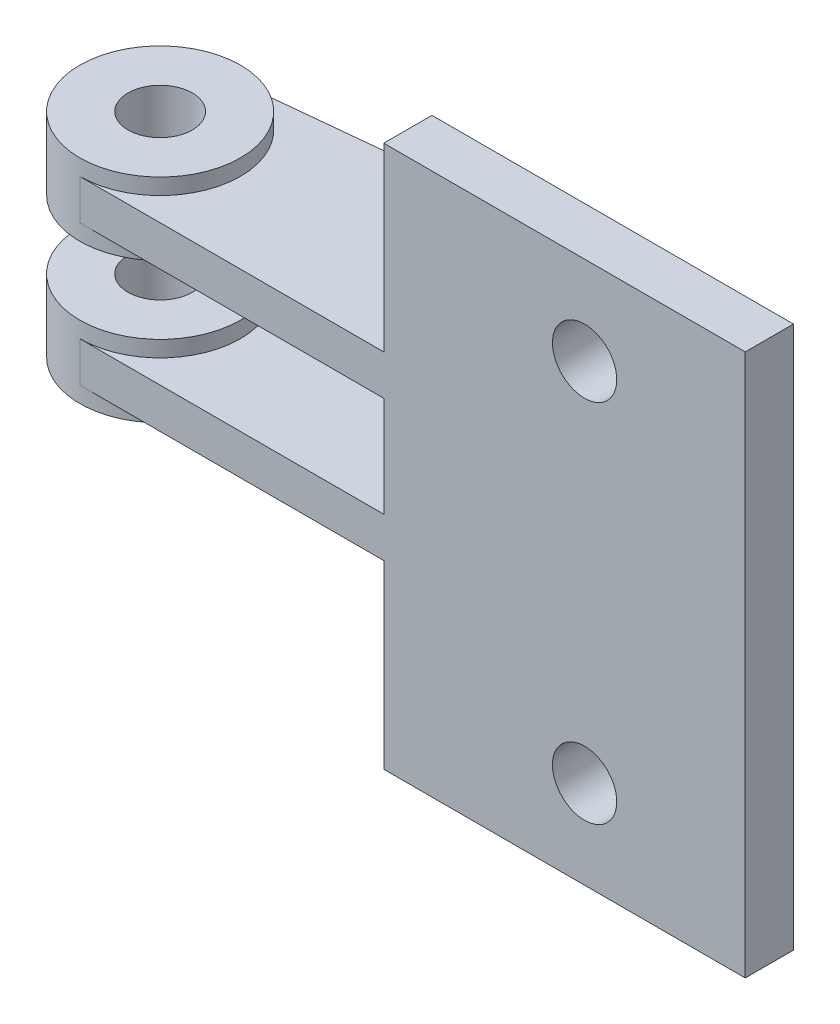
ISO-10303-21;
HEADER;
FILE_DESCRIPTION(('STEP AP214'),'2;1');
FILE_NAME('part.step','',(''),(''),'','','');
FILE_SCHEMA(('AUTOMOTIVE_DESIGN { 1 0 10303 214 1 1 1 1 }'));
ENDSEC;
DATA;
#1=APPLICATION_CONTEXT('core data for automotive mechanical design processes');
#2=APPLICATION_PROTOCOL_DEFINITION('international standard','automotive_design',2000,#1);
#3=PRODUCT_CONTEXT('',#1,'mechanical');
#4=PRODUCT('Part','Part','',(#3));
#5=PRODUCT_RELATED_PRODUCT_CATEGORY('part','',(#4));
#6=PRODUCT_DEFINITION_FORMATION('','',#4);
#7=PRODUCT_DEFINITION_CONTEXT('part definition',#1,'design');
#8=PRODUCT_DEFINITION('design','',#6,#7);
#9=PRODUCT_DEFINITION_SHAPE('','',#8);
#10=(LENGTH_UNIT() NAMED_UNIT(*) SI_UNIT(.MILLI.,.METRE.));
#11=(NAMED_UNIT(*) PLANE_ANGLE_UNIT() SI_UNIT($,.RADIAN.));
#12=(NAMED_UNIT(*) SI_UNIT($,.STERADIAN.) SOLID_ANGLE_UNIT());
#13=UNCERTAINTY_MEASURE_WITH_UNIT(LENGTH_MEASURE(1.E-05),#10,'distance_accuracy_value','');
#14=(GEOMETRIC_REPRESENTATION_CONTEXT(3) GLOBAL_UNCERTAINTY_ASSIGNED_CONTEXT((#13)) GLOBAL_UNIT_ASSIGNED_CONTEXT((#10,
#11,#12)) REPRESENTATION_CONTEXT('',''));
#15=CARTESIAN_POINT('',(0.,0.,0.));
#16=DIRECTION('',(0.,0.,1.));
#17=DIRECTION('',(1.,0.,0.));
#18=AXIS2_PLACEMENT_3D('',#15,#16,#17);
#19=CARTESIAN_POINT('',(-140.672374094552,12.5,0.));
#20=DIRECTION('',(0.,1.,0.));
#21=DIRECTION('',(0.,0.,1.));
#22=AXIS2_PLACEMENT_3D('',#19,#20,#21);
#23=PLANE('',#22);
#24=CARTESIAN_POINT('',(-120.672374094552,12.5,-7.99999999999999));
#25=DIRECTION('',(0.,1.,0.));
#26=DIRECTION('',(0.,0.,1.));
#27=AXIS2_PLACEMENT_3D('',#24,#25,#26);
#28=CIRCLE('',#27,20.);
#29=CARTESIAN_POINT('',(-122.695594955068,12.5,-27.8974012712609));
#30=VERTEX_POINT('',#29);
#31=CARTESIAN_POINT('',(-120.672374094552,12.5,12.));
#32=VERTEX_POINT('',#31);
#33=EDGE_CURVE('E11',#30,#32,#28,.F.);
#34=ORIENTED_EDGE('',*,*,#33,.F.);
#35=DIRECTION('',(-0.994870063563044,0.,0.10116104302579));
#36=VECTOR('',#35,1.);
#37=CARTESIAN_POINT('',(-4.06326518045554,12.5,-39.9602531512327));
#38=LINE('',#37,#36);
#39=CARTESIAN_POINT('',(-3.67237409455184,12.5,-40.));
#40=VERTEX_POINT('',#39);
#41=EDGE_CURVE('E275',#40,#30,#38,.T.);
#42=ORIENTED_EDGE('',*,*,#41,.F.);
#43=DIRECTION('',(-0.772577366580188,0.,-0.634920634920635));
#44=VECTOR('',#43,1.);
#45=CARTESIAN_POINT('',(18.140589569161,12.5,-22.0736390451482));
#46=LINE('',#45,#44);
#47=CARTESIAN_POINT('',(45.,12.5,0.));
#48=VERTEX_POINT('',#47);
#49=EDGE_CURVE('E281',#48,#40,#46,.T.);
#50=ORIENTED_EDGE('',*,*,#49,.F.);
#51=DIRECTION('',(1.,0.,0.));
#52=VECTOR('',#51,1.);
#53=CARTESIAN_POINT('',(-140.672374094552,12.5,0.));
#54=LINE('',#53,#52);
#55=CARTESIAN_POINT('',(-45.,12.5,0.));
#56=VERTEX_POINT('',#55);
#57=EDGE_CURVE('E61',#56,#48,#54,.T.);
#58=ORIENTED_EDGE('',*,*,#57,.F.);
#59=DIRECTION('',(0.,0.,1.));
#60=VECTOR('',#59,1.);
#61=CARTESIAN_POINT('',(-45.,12.5,-40.));
#62=LINE('',#61,#60);
#63=CARTESIAN_POINT('',(-45.,12.5,12.));
#64=VERTEX_POINT('',#63);
#65=EDGE_CURVE('E167',#56,#64,#62,.T.);
#66=ORIENTED_EDGE('',*,*,#65,.T.);
#67=DIRECTION('',(-1.,0.,0.));
#68=VECTOR('',#67,1.);
#69=CARTESIAN_POINT('',(-139.002676874375,12.5,12.));
#70=LINE('',#69,#68);
#71=EDGE_CURVE('E163',#64,#32,#70,.T.);
#72=ORIENTED_EDGE('',*,*,#71,.T.);
#73=EDGE_LOOP('',(#34,#42,#50,#58,#66,#72));
#74=FACE_BOUND('',#73,.T.);
#75=ADVANCED_FACE('F41',(#74),#23,.F.);
#76=CARTESIAN_POINT('',(0.,22.5,0.));
#77=DIRECTION('',(0.,1.,0.));
#78=DIRECTION('',(0.,0.,1.));
#79=AXIS2_PLACEMENT_3D('',#76,#77,#78);
#80=PLANE('',#79);
#81=DIRECTION('',(-0.994870063563044,0.,0.10116104302579));
#82=VECTOR('',#81,1.);
#83=CARTESIAN_POINT('',(-4.06326518045554,22.5,-39.9602531512327));
#84=LINE('',#83,#82);
#85=CARTESIAN_POINT('',(-3.67237409455183,22.5,-40.));
#86=VERTEX_POINT('',#85);
#87=CARTESIAN_POINT('',(-122.695594955068,22.5,-27.8974012712609));
#88=VERTEX_POINT('',#87);
#89=EDGE_CURVE('E270',#86,#88,#84,.T.);
#90=ORIENTED_EDGE('',*,*,#89,.T.);
#91=CARTESIAN_POINT('',(-120.672374094552,22.5,-7.99999999999999));
#92=DIRECTION('',(0.,1.,0.));
#93=DIRECTION('',(0.,0.,1.));
#94=AXIS2_PLACEMENT_3D('',#91,#92,#93);
#95=CIRCLE('',#94,20.);
#96=CARTESIAN_POINT('',(-120.672374094552,22.5,12.));
#97=VERTEX_POINT('',#96);
#98=EDGE_CURVE('E177',#97,#88,#95,.T.);
#99=ORIENTED_EDGE('',*,*,#98,.F.);
#100=DIRECTION('',(-1.,0.,0.));
#101=VECTOR('',#100,1.);
#102=CARTESIAN_POINT('',(0.,22.5,12.));
#103=LINE('',#102,#101);
#104=CARTESIAN_POINT('',(-45.,22.5,12.));
#105=VERTEX_POINT('',#104);
#106=EDGE_CURVE('E161',#105,#97,#103,.T.);
#107=ORIENTED_EDGE('',*,*,#106,.F.);
#108=DIRECTION('',(0.,0.,-1.));
#109=VECTOR('',#108,1.);
#110=CARTESIAN_POINT('',(-45.,22.5,0.));
#111=LINE('',#110,#109);
#112=CARTESIAN_POINT('',(-45.,22.5,0.));
#113=VERTEX_POINT('',#112);
#114=EDGE_CURVE('E279',#105,#113,#111,.T.);
#115=ORIENTED_EDGE('',*,*,#114,.T.);
#116=DIRECTION('',(-1.,0.,0.));
#117=VECTOR('',#116,1.);
#118=CARTESIAN_POINT('',(0.,22.5,0.));
#119=LINE('',#118,#117);
#120=CARTESIAN_POINT('',(45.,22.5,0.));
#121=VERTEX_POINT('',#120);
#122=EDGE_CURVE('E273',#121,#113,#119,.T.);
#123=ORIENTED_EDGE('',*,*,#122,.F.);
#124=DIRECTION('',(-0.772577366580188,0.,-0.634920634920635));
#125=VECTOR('',#124,1.);
#126=CARTESIAN_POINT('',(18.140589569161,22.5,-22.0736390451482));
#127=LINE('',#126,#125);
#128=EDGE_CURVE('E271',#121,#86,#127,.T.);
#129=ORIENTED_EDGE('',*,*,#128,.T.);
#130=EDGE_LOOP('',(#90,#99,#107,#115,#123,#129));
#131=FACE_BOUND('',#130,.T.);
#132=ADVANCED_FACE('F341',(#131),#80,.T.);
#133=CARTESIAN_POINT('',(-140.672374094552,-12.5,0.));
#134=DIRECTION('',(0.,-1.,0.));
#135=DIRECTION('',(0.,0.,-1.));
#136=AXIS2_PLACEMENT_3D('',#133,#134,#135);
#137=PLANE('',#136);
#138=CARTESIAN_POINT('',(-120.672374094552,-12.5,-7.99999999999999));
#139=DIRECTION('',(0.,1.,0.));
#140=DIRECTION('',(0.,0.,1.));
#141=AXIS2_PLACEMENT_3D('',#138,#139,#140);
#142=CIRCLE('',#141,20.);
#143=CARTESIAN_POINT('',(-120.672374094552,-12.5,12.));
#144=VERTEX_POINT('',#143);
#145=CARTESIAN_POINT('',(-122.695594955068,-12.5,-27.8974012712609));
#146=VERTEX_POINT('',#145);
#147=EDGE_CURVE('E308',#144,#146,#142,.T.);
#148=ORIENTED_EDGE('',*,*,#147,.F.);
#149=DIRECTION('',(1.,0.,0.));
#150=VECTOR('',#149,1.);
#151=CARTESIAN_POINT('',(-139.002676874375,-12.5,12.));
#152=LINE('',#151,#150);
#153=CARTESIAN_POINT('',(-45.,-12.5,12.));
#154=VERTEX_POINT('',#153);
#155=EDGE_CURVE('E255',#144,#154,#152,.T.);
#156=ORIENTED_EDGE('',*,*,#155,.T.);
#157=DIRECTION('',(0.,0.,1.));
#158=VECTOR('',#157,1.);
#159=CARTESIAN_POINT('',(-45.,-12.5,-40.));
#160=LINE('',#159,#158);
#161=CARTESIAN_POINT('',(-45.,-12.5,0.));
#162=VERTEX_POINT('',#161);
#163=EDGE_CURVE('E57',#162,#154,#160,.T.);
#164=ORIENTED_EDGE('',*,*,#163,.F.);
#165=DIRECTION('',(1.,0.,0.));
#166=VECTOR('',#165,1.);
#167=CARTESIAN_POINT('',(-140.672374094552,-12.5,0.));
#168=LINE('',#167,#166);
#169=CARTESIAN_POINT('',(45.,-12.5,0.));
#170=VERTEX_POINT('',#169);
#171=EDGE_CURVE('E289',#162,#170,#168,.T.);
#172=ORIENTED_EDGE('',*,*,#171,.T.);
#173=DIRECTION('',(0.772577366580188,0.,0.634920634920635));
#174=VECTOR('',#173,1.);
#175=CARTESIAN_POINT('',(18.140589569161,-12.5,-22.0736390451482));
#176=LINE('',#175,#174);
#177=CARTESIAN_POINT('',(-3.67237409455191,-12.5,-40.));
#178=VERTEX_POINT('',#177);
#179=EDGE_CURVE('E290',#178,#170,#176,.T.);
#180=ORIENTED_EDGE('',*,*,#179,.F.);
#181=DIRECTION('',(0.994870063563044,0.,-0.10116104302579));
#182=VECTOR('',#181,1.);
#183=CARTESIAN_POINT('',(-4.06326518045554,-12.5,-39.9602531512327));
#184=LINE('',#183,#182);
#185=EDGE_CURVE('E282',#146,#178,#184,.T.);
#186=ORIENTED_EDGE('',*,*,#185,.F.);
#187=EDGE_LOOP('',(#148,#156,#164,#172,#180,#186));
#188=FACE_BOUND('',#187,.T.);
#189=ADVANCED_FACE('F347',(#188),#137,.F.);
#190=CARTESIAN_POINT('',(0.,-22.5,0.));
#191=DIRECTION('',(0.,1.,0.));
#192=DIRECTION('',(0.,0.,1.));
#193=AXIS2_PLACEMENT_3D('',#190,#191,#192);
#194=PLANE('',#193);
#195=CARTESIAN_POINT('',(-120.672374094552,-22.5,-7.99999999999999));
#196=DIRECTION('',(0.,1.,0.));
#197=DIRECTION('',(0.,0.,1.));
#198=AXIS2_PLACEMENT_3D('',#195,#196,#197);
#199=CIRCLE('',#198,20.);
#200=CARTESIAN_POINT('',(-122.695594955068,-22.5,-27.8974012712609));
#201=VERTEX_POINT('',#200);
#202=CARTESIAN_POINT('',(-120.672374094552,-22.5,12.));
#203=VERTEX_POINT('',#202);
#204=EDGE_CURVE('E47',#201,#203,#199,.F.);
#205=ORIENTED_EDGE('',*,*,#204,.F.);
#206=DIRECTION('',(-0.994870063563044,0.,0.10116104302579));
#207=VECTOR('',#206,1.);
#208=CARTESIAN_POINT('',(-4.06326518045554,-22.5,-39.9602531512327));
#209=LINE('',#208,#207);
#210=CARTESIAN_POINT('',(-3.67237409455183,-22.5,-40.));
#211=VERTEX_POINT('',#210);
#212=EDGE_CURVE('E242',#211,#201,#209,.T.);
#213=ORIENTED_EDGE('',*,*,#212,.F.);
#214=DIRECTION('',(-0.772577366580188,0.,-0.634920634920635));
#215=VECTOR('',#214,1.);
#216=CARTESIAN_POINT('',(18.140589569161,-22.5,-22.0736390451482));
#217=LINE('',#216,#215);
#218=CARTESIAN_POINT('',(45.,-22.5,0.));
#219=VERTEX_POINT('',#218);
#220=EDGE_CURVE('E264',#219,#211,#217,.T.);
#221=ORIENTED_EDGE('',*,*,#220,.F.);
#222=DIRECTION('',(-1.,0.,0.));
#223=VECTOR('',#222,1.);
#224=CARTESIAN_POINT('',(0.,-22.5,0.));
#225=LINE('',#224,#223);
#226=CARTESIAN_POINT('',(-45.,-22.5,0.));
#227=VERTEX_POINT('',#226);
#228=EDGE_CURVE('E266',#219,#227,#225,.T.);
#229=ORIENTED_EDGE('',*,*,#228,.T.);
#230=DIRECTION('',(0.,0.,-1.));
#231=VECTOR('',#230,1.);
#232=CARTESIAN_POINT('',(-45.,-22.5,0.));
#233=LINE('',#232,#231);
#234=CARTESIAN_POINT('',(-45.,-22.5,12.));
#235=VERTEX_POINT('',#234);
#236=EDGE_CURVE('E247',#235,#227,#233,.T.);
#237=ORIENTED_EDGE('',*,*,#236,.F.);
#238=DIRECTION('',(-1.,0.,0.));
#239=VECTOR('',#238,1.);
#240=CARTESIAN_POINT('',(0.,-22.5,12.));
#241=LINE('',#240,#239);
#242=EDGE_CURVE('E246',#235,#203,#241,.T.);
#243=ORIENTED_EDGE('',*,*,#242,.T.);
#244=EDGE_LOOP('',(#205,#213,#221,#229,#237,#243));
#245=FACE_BOUND('',#244,.T.);
#246=ADVANCED_FACE('F245',(#245),#194,.F.);
#247=CARTESIAN_POINT('',(-120.672374094552,22.5,-7.99999999999999));
#248=DIRECTION('',(0.,-1.,0.));
#249=DIRECTION('',(0.,0.,-1.));
#250=AXIS2_PLACEMENT_3D('',#247,#248,#249);
#251=CYLINDRICAL_SURFACE('',#250,20.);
#252=DIRECTION('',(0.,-1.,0.));
#253=VECTOR('',#252,1.);
#254=CARTESIAN_POINT('',(-122.695594955068,22.5,-27.8974012712609));
#255=LINE('',#254,#253);
#256=EDGE_CURVE('E178',#88,#30,#255,.T.);
#257=ORIENTED_EDGE('',*,*,#256,.T.);
#258=ORIENTED_EDGE('',*,*,#33,.T.);
#259=DIRECTION('',(0.,-1.,0.));
#260=VECTOR('',#259,1.);
#261=CARTESIAN_POINT('',(-120.672374094552,22.5,12.));
#262=LINE('',#261,#260);
#263=EDGE_CURVE('E160',#97,#32,#262,.T.);
#264=ORIENTED_EDGE('',*,*,#263,.F.);
#265=ORIENTED_EDGE('',*,*,#98,.T.);
#266=EDGE_LOOP('',(#257,#258,#264,#265));
#267=FACE_BOUND('',#266,.T.);
#268=CARTESIAN_POINT('',(-120.672374094552,26.5,-7.99999999999999));
#269=DIRECTION('',(0.,1.,0.));
#270=DIRECTION('',(0.,0.,1.));
#271=AXIS2_PLACEMENT_3D('',#268,#269,#270);
#272=CIRCLE('',#271,20.);
#273=CARTESIAN_POINT('',(-120.672374094552,26.5,12.));
#274=VERTEX_POINT('',#273);
#275=EDGE_CURVE('E314',#274,#274,#272,.T.);
#276=ORIENTED_EDGE('',*,*,#275,.F.);
#277=EDGE_LOOP('',(#276));
#278=FACE_BOUND('',#277,.T.);
#279=CARTESIAN_POINT('',(-120.672374094552,8.5,-7.99999999999999));
#280=DIRECTION('',(0.,-1.,0.));
#281=DIRECTION('',(0.,0.,-1.));
#282=AXIS2_PLACEMENT_3D('',#279,#280,#281);
#283=CIRCLE('',#282,20.);
#284=CARTESIAN_POINT('',(-120.672374094552,8.5,-28.));
#285=VERTEX_POINT('',#284);
#286=EDGE_CURVE('E325',#285,#285,#283,.T.);
#287=ORIENTED_EDGE('',*,*,#286,.F.);
#288=EDGE_LOOP('',(#287));
#289=FACE_BOUND('',#288,.T.);
#290=ADVANCED_FACE('F174',(#267,#278,#289),#251,.T.);
#291=CARTESIAN_POINT('',(-4.06326518045554,22.5,-39.9602531512327));
#292=DIRECTION('',(0.10116104302579,0.,0.994870063563044));
#293=DIRECTION('',(0.994870063563044,0.,-0.10116104302579));
#294=AXIS2_PLACEMENT_3D('',#291,#292,#293);
#295=PLANE('',#294);
#296=DIRECTION('',(0.,-1.,0.));
#297=VECTOR('',#296,1.);
#298=CARTESIAN_POINT('',(-3.67237409455183,22.5,-40.));
#299=LINE('',#298,#297);
#300=EDGE_CURVE('E256',#86,#40,#299,.T.);
#301=ORIENTED_EDGE('',*,*,#300,.T.);
#302=ORIENTED_EDGE('',*,*,#41,.T.);
#303=ORIENTED_EDGE('',*,*,#256,.F.);
#304=ORIENTED_EDGE('',*,*,#89,.F.);
#305=EDGE_LOOP('',(#301,#302,#303,#304));
#306=FACE_BOUND('',#305,.T.);
#307=ADVANCED_FACE('F379',(#306),#295,.F.);
#308=CARTESIAN_POINT('',(18.140589569161,22.5,-22.0736390451482));
#309=DIRECTION('',(-0.634920634920635,0.,0.772577366580188));
#310=DIRECTION('',(0.772577366580188,0.,0.634920634920635));
#311=AXIS2_PLACEMENT_3D('',#308,#309,#310);
#312=PLANE('',#311);
#313=DIRECTION('',(0.,-1.,0.));
#314=VECTOR('',#313,1.);
#315=CARTESIAN_POINT('',(45.,22.5,0.));
#316=LINE('',#315,#314);
#317=EDGE_CURVE('E254',#121,#48,#316,.T.);
#318=ORIENTED_EDGE('',*,*,#317,.T.);
#319=ORIENTED_EDGE('',*,*,#49,.T.);
#320=ORIENTED_EDGE('',*,*,#300,.F.);
#321=ORIENTED_EDGE('',*,*,#128,.F.);
#322=EDGE_LOOP('',(#318,#319,#320,#321));
#323=FACE_BOUND('',#322,.T.);
#324=ADVANCED_FACE('F375',(#323),#312,.F.);
#325=CARTESIAN_POINT('',(-120.672374094552,22.5,-7.99999999999999));
#326=DIRECTION('',(0.,-1.,0.));
#327=DIRECTION('',(0.,0.,-1.));
#328=AXIS2_PLACEMENT_3D('',#325,#326,#327);
#329=CYLINDRICAL_SURFACE('',#328,8.00000000000001);
#330=CARTESIAN_POINT('',(-120.672374094552,26.5,-7.99999999999999));
#331=DIRECTION('',(0.,1.,0.));
#332=DIRECTION('',(0.,0.,1.));
#333=AXIS2_PLACEMENT_3D('',#330,#331,#332);
#334=CIRCLE('',#333,8.00000000000001);
#335=CARTESIAN_POINT('',(-120.672374094552,26.5,-16.));
#336=VERTEX_POINT('',#335);
#337=EDGE_CURVE('E320',#336,#336,#334,.T.);
#338=CARTESIAN_POINT('',(-120.672374094552,8.5,-7.99999999999999));
#339=DIRECTION('',(0.,-1.,0.));
#340=DIRECTION('',(0.,0.,-1.));
#341=AXIS2_PLACEMENT_3D('',#338,#339,#340);
#342=CIRCLE('',#341,7.99999999999998);
#343=CARTESIAN_POINT('',(-120.672374094552,8.5,-16.));
#344=VERTEX_POINT('',#343);
#345=EDGE_CURVE('E323',#344,#344,#342,.T.);
#346=CARTESIAN_POINT('',(-120.672374094552,26.5,-16.));
#347=CARTESIAN_POINT('',(-120.672374094552,26.3125,-16.));
#348=CARTESIAN_POINT('',(-120.672374094552,26.125,-16.));
#349=CARTESIAN_POINT('',(-120.672374094552,25.75,-16.));
#350=CARTESIAN_POINT('',(-120.672374094552,25.5625,-16.));
#351=CARTESIAN_POINT('',(-120.672374094552,25.1875,-16.));
#352=CARTESIAN_POINT('',(-120.672374094552,25.,-16.));
#353=CARTESIAN_POINT('',(-120.672374094552,24.625,-16.));
#354=CARTESIAN_POINT('',(-120.672374094552,24.4375,-16.));
#355=CARTESIAN_POINT('',(-120.672374094552,24.0625,-16.));
#356=CARTESIAN_POINT('',(-120.672374094552,23.875,-16.));
#357=CARTESIAN_POINT('',(-120.672374094552,23.5,-16.));
#358=CARTESIAN_POINT('',(-120.672374094552,23.3125,-16.));
#359=CARTESIAN_POINT('',(-120.672374094552,22.9375,-16.));
#360=CARTESIAN_POINT('',(-120.672374094552,22.75,-16.));
#361=CARTESIAN_POINT('',(-120.672374094552,22.375,-16.));
#362=CARTESIAN_POINT('',(-120.672374094552,22.1875,-16.));
#363=CARTESIAN_POINT('',(-120.672374094552,21.8125,-16.));
#364=CARTESIAN_POINT('',(-120.672374094552,21.625,-16.));
#365=CARTESIAN_POINT('',(-120.672374094552,21.25,-16.));
#366=CARTESIAN_POINT('',(-120.672374094552,21.0625,-16.));
#367=CARTESIAN_POINT('',(-120.672374094552,20.6875,-16.));
#368=CARTESIAN_POINT('',(-120.672374094552,20.5,-16.));
#369=CARTESIAN_POINT('',(-120.672374094552,20.125,-16.));
#370=CARTESIAN_POINT('',(-120.672374094552,19.9375,-16.));
#371=CARTESIAN_POINT('',(-120.672374094552,19.5625,-16.));
#372=CARTESIAN_POINT('',(-120.672374094552,19.375,-16.));
#373=CARTESIAN_POINT('',(-120.672374094552,19.,-16.));
#374=CARTESIAN_POINT('',(-120.672374094552,18.8125,-16.));
#375=CARTESIAN_POINT('',(-120.672374094552,18.4375,-16.));
#376=CARTESIAN_POINT('',(-120.672374094552,18.25,-16.));
#377=CARTESIAN_POINT('',(-120.672374094552,17.875,-16.));
#378=CARTESIAN_POINT('',(-120.672374094552,17.6875,-16.));
#379=CARTESIAN_POINT('',(-120.672374094552,17.3125,-16.));
#380=CARTESIAN_POINT('',(-120.672374094552,17.125,-16.));
#381=CARTESIAN_POINT('',(-120.672374094552,16.75,-16.));
#382=CARTESIAN_POINT('',(-120.672374094552,16.5625,-16.));
#383=CARTESIAN_POINT('',(-120.672374094552,16.1875,-16.));
#384=CARTESIAN_POINT('',(-120.672374094552,16.,-16.));
#385=CARTESIAN_POINT('',(-120.672374094552,15.625,-16.));
#386=CARTESIAN_POINT('',(-120.672374094552,15.4375,-16.));
#387=CARTESIAN_POINT('',(-120.672374094552,15.0625,-16.));
#388=CARTESIAN_POINT('',(-120.672374094552,14.875,-16.));
#389=CARTESIAN_POINT('',(-120.672374094552,14.5,-16.));
#390=CARTESIAN_POINT('',(-120.672374094552,14.3125,-16.));
#391=CARTESIAN_POINT('',(-120.672374094552,13.9375,-16.));
#392=CARTESIAN_POINT('',(-120.672374094552,13.75,-16.));
#393=CARTESIAN_POINT('',(-120.672374094552,13.375,-16.));
#394=CARTESIAN_POINT('',(-120.672374094552,13.1875,-16.));
#395=CARTESIAN_POINT('',(-120.672374094552,12.8125,-16.));
#396=CARTESIAN_POINT('',(-120.672374094552,12.625,-16.));
#397=CARTESIAN_POINT('',(-120.672374094552,12.25,-16.));
#398=CARTESIAN_POINT('',(-120.672374094552,12.0625,-16.));
#399=CARTESIAN_POINT('',(-120.672374094552,11.6875,-16.));
#400=CARTESIAN_POINT('',(-120.672374094552,11.5,-16.));
#401=CARTESIAN_POINT('',(-120.672374094552,11.125,-16.));
#402=CARTESIAN_POINT('',(-120.672374094552,10.9375,-16.));
#403=CARTESIAN_POINT('',(-120.672374094552,10.5625,-16.));
#404=CARTESIAN_POINT('',(-120.672374094552,10.375,-16.));
#405=CARTESIAN_POINT('',(-120.672374094552,10.,-16.));
#406=CARTESIAN_POINT('',(-120.672374094552,9.8125,-16.));
#407=CARTESIAN_POINT('',(-120.672374094552,9.4375,-16.));
#408=CARTESIAN_POINT('',(-120.672374094552,9.25,-16.));
#409=CARTESIAN_POINT('',(-120.672374094552,8.875,-16.));
#410=CARTESIAN_POINT('',(-120.672374094552,8.6875,-16.));
#411=CARTESIAN_POINT('',(-120.672374094552,8.5,-16.));
#412=B_SPLINE_CURVE_WITH_KNOTS('',3,(#346,#347,#348,#349,#350,#351,#352,#353,#354,#355,#356,
#357,#358,#359,#360,#361,#362,#363,#364,#365,#366,#367,#368,#369,#370,#371,#372,#373,#374,#375,
#376,#377,#378,#379,#380,#381,#382,#383,#384,#385,#386,#387,#388,#389,#390,#391,#392,#393,#394,
#395,#396,#397,#398,#399,#400,#401,#402,#403,#404,#405,#406,#407,#408,#409,#410,#411),
.UNSPECIFIED.,.F.,.F.,(4,2,2,2,2,2,2,2,2,2,2,2,2,2,2,2,2,2,2,2,2,2,2,2,2,2,2,2,2,2,2,2,4),(0.,
0.5625,1.125,1.6875,2.25,2.8125,3.375,3.9375,4.5,5.0625,5.625,6.1875,6.75,7.3125,7.875,8.4375,
9.,9.5625,10.125,10.6875,11.25,11.8125,12.375,12.9375,13.5,14.0625,14.625,15.1875,15.75,16.3125,
16.875,17.4375,18.),.UNSPECIFIED.);
#413=EDGE_CURVE('BSEAM329',#336,#344,#412,.T.);
#414=ORIENTED_EDGE('',*,*,#337,.T.);
#415=ORIENTED_EDGE('',*,*,#345,.T.);
#416=ORIENTED_EDGE('',*,*,#413,.T.);
#417=ORIENTED_EDGE('',*,*,#413,.F.);
#418=EDGE_LOOP('',(#414,#416,#415,#417));
#419=FACE_BOUND('',#418,.T.);
#420=ADVANCED_FACE('F329',(#419),#329,.F.);
#421=CARTESIAN_POINT('',(-45.,-67.5,12.));
#422=DIRECTION('',(1.,0.,0.));
#423=DIRECTION('',(0.,0.,-1.));
#424=AXIS2_PLACEMENT_3D('',#421,#422,#423);
#425=PLANE('',#424);
#426=ORIENTED_EDGE('',*,*,#236,.T.);
#427=DIRECTION('',(0.,-1.,0.));
#428=VECTOR('',#427,1.);
#429=CARTESIAN_POINT('',(-45.,-67.5,0.));
#430=LINE('',#429,#428);
#431=CARTESIAN_POINT('',(-45.,-67.5,0.));
#432=VERTEX_POINT('',#431);
#433=EDGE_CURVE('E215',#227,#432,#430,.T.);
#434=ORIENTED_EDGE('',*,*,#433,.T.);
#435=DIRECTION('',(0.,0.,-1.));
#436=VECTOR('',#435,1.);
#437=CARTESIAN_POINT('',(-45.,-67.5,12.));
#438=LINE('',#437,#436);
#439=CARTESIAN_POINT('',(-45.,-67.5,12.));
#440=VERTEX_POINT('',#439);
#441=EDGE_CURVE('E219',#440,#432,#438,.T.);
#442=ORIENTED_EDGE('',*,*,#441,.F.);
#443=DIRECTION('',(0.,-1.,0.));
#444=VECTOR('',#443,1.);
#445=CARTESIAN_POINT('',(-45.,-67.5,12.));
#446=LINE('',#445,#444);
#447=EDGE_CURVE('E197',#235,#440,#446,.T.);
#448=ORIENTED_EDGE('',*,*,#447,.F.);
#449=EDGE_LOOP('',(#426,#434,#442,#448));
#450=FACE_BOUND('',#449,.T.);
#451=ADVANCED_FACE('F404',(#450),#425,.F.);
#452=CARTESIAN_POINT('',(0.,0.,0.));
#453=DIRECTION('',(0.,0.,-1.));
#454=DIRECTION('',(-1.,0.,0.));
#455=AXIS2_PLACEMENT_3D('',#452,#453,#454);
#456=PLANE('',#455);
#457=CARTESIAN_POINT('',(5.,-45.5,0.));
#458=DIRECTION('',(0.,0.,-1.));
#459=DIRECTION('',(-1.,0.,0.));
#460=AXIS2_PLACEMENT_3D('',#457,#458,#459);
#461=CIRCLE('',#460,8.);
#462=CARTESIAN_POINT('',(-3.,-45.5,0.));
#463=VERTEX_POINT('',#462);
#464=EDGE_CURVE('E229',#463,#463,#461,.T.);
#465=ORIENTED_EDGE('',*,*,#464,.F.);
#466=EDGE_LOOP('',(#465));
#467=FACE_BOUND('',#466,.T.);
#468=ORIENTED_EDGE('',*,*,#433,.F.);
#469=ORIENTED_EDGE('',*,*,#228,.F.);
#470=DIRECTION('',(0.,1.,0.));
#471=VECTOR('',#470,1.);
#472=CARTESIAN_POINT('',(45.,-67.5,0.));
#473=LINE('',#472,#471);
#474=CARTESIAN_POINT('',(45.,-67.5,0.));
#475=VERTEX_POINT('',#474);
#476=EDGE_CURVE('E207',#475,#219,#473,.T.);
#477=ORIENTED_EDGE('',*,*,#476,.F.);
#478=DIRECTION('',(1.,0.,0.));
#479=VECTOR('',#478,1.);
#480=CARTESIAN_POINT('',(-45.,-67.5,0.));
#481=LINE('',#480,#479);
#482=EDGE_CURVE('E196',#432,#475,#481,.T.);
#483=ORIENTED_EDGE('',*,*,#482,.F.);
#484=EDGE_LOOP('',(#468,#469,#477,#483));
#485=FACE_BOUND('',#484,.T.);
#486=ADVANCED_FACE('F398',(#467,#485),#456,.T.);
#487=CARTESIAN_POINT('',(45.,-67.5,12.));
#488=DIRECTION('',(-1.,0.,0.));
#489=DIRECTION('',(0.,0.,1.));
#490=AXIS2_PLACEMENT_3D('',#487,#488,#489);
#491=PLANE('',#490);
#492=ORIENTED_EDGE('',*,*,#476,.T.);
#493=EDGE_CURVE('E253',#170,#219,#316,.T.);
#494=ORIENTED_EDGE('',*,*,#493,.F.);
#495=DIRECTION('',(0.,-1.,0.));
#496=VECTOR('',#495,1.);
#497=CARTESIAN_POINT('',(45.,12.5,0.));
#498=LINE('',#497,#496);
#499=EDGE_CURVE('E292',#48,#170,#498,.T.);
#500=ORIENTED_EDGE('',*,*,#499,.F.);
#501=ORIENTED_EDGE('',*,*,#317,.F.);
#502=CARTESIAN_POINT('',(45.,67.5,0.));
#503=VERTEX_POINT('',#502);
#504=EDGE_CURVE('E208',#121,#503,#473,.T.);
#505=ORIENTED_EDGE('',*,*,#504,.T.);
#506=DIRECTION('',(0.,0.,-1.));
#507=VECTOR('',#506,1.);
#508=CARTESIAN_POINT('',(45.,67.5,12.));
#509=LINE('',#508,#507);
#510=CARTESIAN_POINT('',(45.,67.5,12.));
#511=VERTEX_POINT('',#510);
#512=EDGE_CURVE('E224',#511,#503,#509,.T.);
#513=ORIENTED_EDGE('',*,*,#512,.F.);
#514=DIRECTION('',(0.,1.,0.));
#515=VECTOR('',#514,1.);
#516=CARTESIAN_POINT('',(45.,-67.5,12.));
#517=LINE('',#516,#515);
#518=CARTESIAN_POINT('',(45.,-67.5,12.));
#519=VERTEX_POINT('',#518);
#520=EDGE_CURVE('E191',#519,#511,#517,.T.);
#521=ORIENTED_EDGE('',*,*,#520,.F.);
#522=DIRECTION('',(0.,0.,-1.));
#523=VECTOR('',#522,1.);
#524=CARTESIAN_POINT('',(45.,-67.5,12.));
#525=LINE('',#524,#523);
#526=EDGE_CURVE('E204',#519,#475,#525,.T.);
#527=ORIENTED_EDGE('',*,*,#526,.T.);
#528=EDGE_LOOP('',(#492,#494,#500,#501,#505,#513,#521,#527));
#529=FACE_BOUND('',#528,.T.);
#530=ADVANCED_FACE('F43',(#529),#491,.F.);
#531=CARTESIAN_POINT('',(-45.,67.5,12.));
#532=DIRECTION('',(0.,-1.,0.));
#533=DIRECTION('',(0.,0.,-1.));
#534=AXIS2_PLACEMENT_3D('',#531,#532,#533);
#535=PLANE('',#534);
#536=DIRECTION('',(-1.,0.,0.));
#537=VECTOR('',#536,1.);
#538=CARTESIAN_POINT('',(-45.,67.5,0.));
#539=LINE('',#538,#537);
#540=CARTESIAN_POINT('',(-45.,67.5,0.));
#541=VERTEX_POINT('',#540);
#542=EDGE_CURVE('E209',#503,#541,#539,.T.);
#543=ORIENTED_EDGE('',*,*,#542,.T.);
#544=DIRECTION('',(0.,0.,-1.));
#545=VECTOR('',#544,1.);
#546=CARTESIAN_POINT('',(-45.,67.5,12.));
#547=LINE('',#546,#545);
#548=CARTESIAN_POINT('',(-45.,67.5,12.));
#549=VERTEX_POINT('',#548);
#550=EDGE_CURVE('E225',#549,#541,#547,.T.);
#551=ORIENTED_EDGE('',*,*,#550,.F.);
#552=DIRECTION('',(-1.,0.,0.));
#553=VECTOR('',#552,1.);
#554=CARTESIAN_POINT('',(-45.,67.5,12.));
#555=LINE('',#554,#553);
#556=EDGE_CURVE('E200',#511,#549,#555,.T.);
#557=ORIENTED_EDGE('',*,*,#556,.F.);
#558=ORIENTED_EDGE('',*,*,#512,.T.);
#559=EDGE_LOOP('',(#543,#551,#557,#558));
#560=FACE_BOUND('',#559,.T.);
#561=ADVANCED_FACE('F405',(#560),#535,.F.);
#562=EDGE_CURVE('E214',#541,#113,#430,.T.);
#563=ORIENTED_EDGE('',*,*,#562,.T.);
#564=ORIENTED_EDGE('',*,*,#114,.F.);
#565=EDGE_CURVE('E203',#549,#105,#446,.T.);
#566=ORIENTED_EDGE('',*,*,#565,.F.);
#567=ORIENTED_EDGE('',*,*,#550,.T.);
#568=EDGE_LOOP('',(#563,#564,#566,#567));
#569=FACE_BOUND('',#568,.T.);
#570=ADVANCED_FACE('F397',(#569),#425,.F.);
#571=CARTESIAN_POINT('',(-45.,-67.5,12.));
#572=DIRECTION('',(0.,1.,0.));
#573=DIRECTION('',(0.,0.,1.));
#574=AXIS2_PLACEMENT_3D('',#571,#572,#573);
#575=PLANE('',#574);
#576=ORIENTED_EDGE('',*,*,#482,.T.);
#577=ORIENTED_EDGE('',*,*,#526,.F.);
#578=DIRECTION('',(1.,0.,0.));
#579=VECTOR('',#578,1.);
#580=CARTESIAN_POINT('',(-45.,-67.5,12.));
#581=LINE('',#580,#579);
#582=EDGE_CURVE('E201',#440,#519,#581,.T.);
#583=ORIENTED_EDGE('',*,*,#582,.F.);
#584=ORIENTED_EDGE('',*,*,#441,.T.);
#585=EDGE_LOOP('',(#576,#577,#583,#584));
#586=FACE_BOUND('',#585,.T.);
#587=ADVANCED_FACE('F393',(#586),#575,.F.);
#588=CARTESIAN_POINT('',(0.,0.,12.));
#589=DIRECTION('',(0.,0.,-1.));
#590=DIRECTION('',(-1.,0.,0.));
#591=AXIS2_PLACEMENT_3D('',#588,#589,#590);
#592=PLANE('',#591);
#593=CARTESIAN_POINT('',(5.,-45.5,12.));
#594=DIRECTION('',(0.,0.,1.));
#595=DIRECTION('',(1.,0.,0.));
#596=AXIS2_PLACEMENT_3D('',#593,#594,#595);
#597=CIRCLE('',#596,8.);
#598=CARTESIAN_POINT('',(13.,-45.5,12.));
#599=VERTEX_POINT('',#598);
#600=EDGE_CURVE('E187',#599,#599,#597,.T.);
#601=ORIENTED_EDGE('',*,*,#600,.F.);
#602=EDGE_LOOP('',(#601));
#603=FACE_BOUND('',#602,.T.);
#604=CARTESIAN_POINT('',(5.,45.5,12.));
#605=DIRECTION('',(0.,0.,1.));
#606=DIRECTION('',(1.,0.,0.));
#607=AXIS2_PLACEMENT_3D('',#604,#605,#606);
#608=CIRCLE('',#607,8.);
#609=CARTESIAN_POINT('',(13.,45.5,12.));
#610=VERTEX_POINT('',#609);
#611=EDGE_CURVE('E182',#610,#610,#608,.T.);
#612=ORIENTED_EDGE('',*,*,#611,.F.);
#613=EDGE_LOOP('',(#612));
#614=FACE_BOUND('',#613,.T.);
#615=ORIENTED_EDGE('',*,*,#263,.T.);
#616=ORIENTED_EDGE('',*,*,#71,.F.);
#617=DIRECTION('',(0.,1.,0.));
#618=VECTOR('',#617,1.);
#619=CARTESIAN_POINT('',(-45.,12.5,12.));
#620=LINE('',#619,#618);
#621=EDGE_CURVE('E175',#154,#64,#620,.T.);
#622=ORIENTED_EDGE('',*,*,#621,.F.);
#623=ORIENTED_EDGE('',*,*,#155,.F.);
#624=EDGE_CURVE('E168',#144,#203,#262,.T.);
#625=ORIENTED_EDGE('',*,*,#624,.T.);
#626=ORIENTED_EDGE('',*,*,#242,.F.);
#627=ORIENTED_EDGE('',*,*,#447,.T.);
#628=ORIENTED_EDGE('',*,*,#582,.T.);
#629=ORIENTED_EDGE('',*,*,#520,.T.);
#630=ORIENTED_EDGE('',*,*,#556,.T.);
#631=ORIENTED_EDGE('',*,*,#565,.T.);
#632=ORIENTED_EDGE('',*,*,#106,.T.);
#633=EDGE_LOOP('',(#615,#616,#622,#623,#625,#626,#627,#628,#629,#630,#631,#632));
#634=FACE_BOUND('',#633,.T.);
#635=ADVANCED_FACE('F157',(#603,#614,#634),#592,.F.);
#636=ORIENTED_EDGE('',*,*,#122,.T.);
#637=ORIENTED_EDGE('',*,*,#562,.F.);
#638=ORIENTED_EDGE('',*,*,#542,.F.);
#639=ORIENTED_EDGE('',*,*,#504,.F.);
#640=EDGE_LOOP('',(#636,#637,#638,#639));
#641=FACE_BOUND('',#640,.T.);
#642=CARTESIAN_POINT('',(5.,45.5,0.));
#643=DIRECTION('',(0.,0.,-1.));
#644=DIRECTION('',(-1.,0.,0.));
#645=AXIS2_PLACEMENT_3D('',#642,#643,#644);
#646=CIRCLE('',#645,8.);
#647=CARTESIAN_POINT('',(-3.,45.5,0.));
#648=VERTEX_POINT('',#647);
#649=EDGE_CURVE('E195',#648,#648,#646,.T.);
#650=ORIENTED_EDGE('',*,*,#649,.F.);
#651=EDGE_LOOP('',(#650));
#652=FACE_BOUND('',#651,.T.);
#653=ADVANCED_FACE('F390',(#641,#652),#456,.T.);
#654=CARTESIAN_POINT('',(5.,45.5,-10.));
#655=DIRECTION('',(0.,0.,1.));
#656=DIRECTION('',(1.,0.,0.));
#657=AXIS2_PLACEMENT_3D('',#654,#655,#656);
#658=CYLINDRICAL_SURFACE('',#657,8.);
#659=ORIENTED_EDGE('',*,*,#649,.T.);
#660=EDGE_LOOP('',(#659));
#661=FACE_BOUND('',#660,.T.);
#662=ORIENTED_EDGE('',*,*,#611,.T.);
#663=EDGE_LOOP('',(#662));
#664=FACE_BOUND('',#663,.T.);
#665=ADVANCED_FACE('F384',(#661,#664),#658,.F.);
#666=CARTESIAN_POINT('',(5.,-45.5,-10.));
#667=DIRECTION('',(0.,0.,1.));
#668=DIRECTION('',(1.,0.,0.));
#669=AXIS2_PLACEMENT_3D('',#666,#667,#668);
#670=CYLINDRICAL_SURFACE('',#669,8.);
#671=ORIENTED_EDGE('',*,*,#464,.T.);
#672=EDGE_LOOP('',(#671));
#673=FACE_BOUND('',#672,.T.);
#674=ORIENTED_EDGE('',*,*,#600,.T.);
#675=EDGE_LOOP('',(#674));
#676=FACE_BOUND('',#675,.T.);
#677=ADVANCED_FACE('F377',(#673,#676),#670,.F.);
#678=EDGE_CURVE('E164',#146,#201,#255,.T.);
#679=ORIENTED_EDGE('',*,*,#678,.F.);
#680=ORIENTED_EDGE('',*,*,#185,.T.);
#681=EDGE_CURVE('E261',#178,#211,#299,.T.);
#682=ORIENTED_EDGE('',*,*,#681,.T.);
#683=ORIENTED_EDGE('',*,*,#212,.T.);
#684=EDGE_LOOP('',(#679,#680,#682,#683));
#685=FACE_BOUND('',#684,.T.);
#686=ADVANCED_FACE('F374',(#685),#295,.F.);
#687=ORIENTED_EDGE('',*,*,#624,.F.);
#688=ORIENTED_EDGE('',*,*,#147,.T.);
#689=ORIENTED_EDGE('',*,*,#678,.T.);
#690=ORIENTED_EDGE('',*,*,#204,.T.);
#691=EDGE_LOOP('',(#687,#688,#689,#690));
#692=FACE_BOUND('',#691,.T.);
#693=CARTESIAN_POINT('',(-120.672374094552,-26.5,-7.99999999999999));
#694=DIRECTION('',(0.,-1.,0.));
#695=DIRECTION('',(0.,0.,-1.));
#696=AXIS2_PLACEMENT_3D('',#693,#694,#695);
#697=CIRCLE('',#696,20.);
#698=CARTESIAN_POINT('',(-120.672374094552,-26.5,-28.));
#699=VERTEX_POINT('',#698);
#700=EDGE_CURVE('E301',#699,#699,#697,.T.);
#701=ORIENTED_EDGE('',*,*,#700,.F.);
#702=EDGE_LOOP('',(#701));
#703=FACE_BOUND('',#702,.T.);
#704=CARTESIAN_POINT('',(-120.672374094552,-8.5,-7.99999999999999));
#705=DIRECTION('',(0.,1.,0.));
#706=DIRECTION('',(0.,0.,1.));
#707=AXIS2_PLACEMENT_3D('',#704,#705,#706);
#708=CIRCLE('',#707,20.);
#709=CARTESIAN_POINT('',(-120.672374094552,-8.5,12.));
#710=VERTEX_POINT('',#709);
#711=EDGE_CURVE('E310',#710,#710,#708,.T.);
#712=ORIENTED_EDGE('',*,*,#711,.F.);
#713=EDGE_LOOP('',(#712));
#714=FACE_BOUND('',#713,.T.);
#715=ADVANCED_FACE('F232',(#692,#703,#714),#251,.T.);
#716=ORIENTED_EDGE('',*,*,#681,.F.);
#717=ORIENTED_EDGE('',*,*,#179,.T.);
#718=ORIENTED_EDGE('',*,*,#493,.T.);
#719=ORIENTED_EDGE('',*,*,#220,.T.);
#720=EDGE_LOOP('',(#716,#717,#718,#719));
#721=FACE_BOUND('',#720,.T.);
#722=ADVANCED_FACE('F370',(#721),#312,.F.);
#723=CARTESIAN_POINT('',(-120.672374094552,-26.5,-7.99999999999999));
#724=DIRECTION('',(0.,-1.,0.));
#725=DIRECTION('',(0.,0.,-1.));
#726=AXIS2_PLACEMENT_3D('',#723,#724,#725);
#727=CIRCLE('',#726,8.00000000000001);
#728=CARTESIAN_POINT('',(-120.672374094552,-26.5,-16.));
#729=VERTEX_POINT('',#728);
#730=EDGE_CURVE('E302',#729,#729,#727,.T.);
#731=CARTESIAN_POINT('',(-120.672374094552,-8.5,-7.99999999999999));
#732=DIRECTION('',(0.,1.,0.));
#733=DIRECTION('',(0.,0.,1.));
#734=AXIS2_PLACEMENT_3D('',#731,#732,#733);
#735=CIRCLE('',#734,8.00000000000001);
#736=CARTESIAN_POINT('',(-120.672374094552,-8.5,-16.));
#737=VERTEX_POINT('',#736);
#738=EDGE_CURVE('E309',#737,#737,#735,.T.);
#739=CARTESIAN_POINT('',(-120.672374094552,-26.5,-16.));
#740=CARTESIAN_POINT('',(-120.672374094552,-26.3125,-16.));
#741=CARTESIAN_POINT('',(-120.672374094552,-26.125,-16.));
#742=CARTESIAN_POINT('',(-120.672374094552,-25.75,-16.));
#743=CARTESIAN_POINT('',(-120.672374094552,-25.5625,-16.));
#744=CARTESIAN_POINT('',(-120.672374094552,-25.1875,-16.));
#745=CARTESIAN_POINT('',(-120.672374094552,-25.,-16.));
#746=CARTESIAN_POINT('',(-120.672374094552,-24.625,-16.));
#747=CARTESIAN_POINT('',(-120.672374094552,-24.4375,-16.));
#748=CARTESIAN_POINT('',(-120.672374094552,-24.0625,-16.));
#749=CARTESIAN_POINT('',(-120.672374094552,-23.875,-16.));
#750=CARTESIAN_POINT('',(-120.672374094552,-23.5,-16.));
#751=CARTESIAN_POINT('',(-120.672374094552,-23.3125,-16.));
#752=CARTESIAN_POINT('',(-120.672374094552,-22.9375,-16.));
#753=CARTESIAN_POINT('',(-120.672374094552,-22.75,-16.));
#754=CARTESIAN_POINT('',(-120.672374094552,-22.375,-16.));
#755=CARTESIAN_POINT('',(-120.672374094552,-22.1875,-16.));
#756=CARTESIAN_POINT('',(-120.672374094552,-21.8125,-16.));
#757=CARTESIAN_POINT('',(-120.672374094552,-21.625,-16.));
#758=CARTESIAN_POINT('',(-120.672374094552,-21.25,-16.));
#759=CARTESIAN_POINT('',(-120.672374094552,-21.0625,-16.));
#760=CARTESIAN_POINT('',(-120.672374094552,-20.6875,-16.));
#761=CARTESIAN_POINT('',(-120.672374094552,-20.5,-16.));
#762=CARTESIAN_POINT('',(-120.672374094552,-20.125,-16.));
#763=CARTESIAN_POINT('',(-120.672374094552,-19.9375,-16.));
#764=CARTESIAN_POINT('',(-120.672374094552,-19.5625,-16.));
#765=CARTESIAN_POINT('',(-120.672374094552,-19.375,-16.));
#766=CARTESIAN_POINT('',(-120.672374094552,-19.,-16.));
#767=CARTESIAN_POINT('',(-120.672374094552,-18.8125,-16.));
#768=CARTESIAN_POINT('',(-120.672374094552,-18.4375,-16.));
#769=CARTESIAN_POINT('',(-120.672374094552,-18.25,-16.));
#770=CARTESIAN_POINT('',(-120.672374094552,-17.875,-16.));
#771=CARTESIAN_POINT('',(-120.672374094552,-17.6875,-16.));
#772=CARTESIAN_POINT('',(-120.672374094552,-17.3125,-16.));
#773=CARTESIAN_POINT('',(-120.672374094552,-17.125,-16.));
#774=CARTESIAN_POINT('',(-120.672374094552,-16.75,-16.));
#775=CARTESIAN_POINT('',(-120.672374094552,-16.5625,-16.));
#776=CARTESIAN_POINT('',(-120.672374094552,-16.1875,-16.));
#777=CARTESIAN_POINT('',(-120.672374094552,-16.,-16.));
#778=CARTESIAN_POINT('',(-120.672374094552,-15.625,-16.));
#779=CARTESIAN_POINT('',(-120.672374094552,-15.4375,-16.));
#780=CARTESIAN_POINT('',(-120.672374094552,-15.0625,-16.));
#781=CARTESIAN_POINT('',(-120.672374094552,-14.875,-16.));
#782=CARTESIAN_POINT('',(-120.672374094552,-14.5,-16.));
#783=CARTESIAN_POINT('',(-120.672374094552,-14.3125,-16.));
#784=CARTESIAN_POINT('',(-120.672374094552,-13.9375,-16.));
#785=CARTESIAN_POINT('',(-120.672374094552,-13.75,-16.));
#786=CARTESIAN_POINT('',(-120.672374094552,-13.375,-16.));
#787=CARTESIAN_POINT('',(-120.672374094552,-13.1875,-16.));
#788=CARTESIAN_POINT('',(-120.672374094552,-12.8125,-16.));
#789=CARTESIAN_POINT('',(-120.672374094552,-12.625,-16.));
#790=CARTESIAN_POINT('',(-120.672374094552,-12.25,-16.));
#791=CARTESIAN_POINT('',(-120.672374094552,-12.0625,-16.));
#792=CARTESIAN_POINT('',(-120.672374094552,-11.6875,-16.));
#793=CARTESIAN_POINT('',(-120.672374094552,-11.5,-16.));
#794=CARTESIAN_POINT('',(-120.672374094552,-11.125,-16.));
#795=CARTESIAN_POINT('',(-120.672374094552,-10.9375,-16.));
#796=CARTESIAN_POINT('',(-120.672374094552,-10.5625,-16.));
#797=CARTESIAN_POINT('',(-120.672374094552,-10.375,-16.));
#798=CARTESIAN_POINT('',(-120.672374094552,-10.,-16.));
#799=CARTESIAN_POINT('',(-120.672374094552,-9.8125,-16.));
#800=CARTESIAN_POINT('',(-120.672374094552,-9.4375,-16.));
#801=CARTESIAN_POINT('',(-120.672374094552,-9.25,-16.));
#802=CARTESIAN_POINT('',(-120.672374094552,-8.875,-16.));
#803=CARTESIAN_POINT('',(-120.672374094552,-8.6875,-16.));
#804=CARTESIAN_POINT('',(-120.672374094552,-8.5,-16.));
#805=B_SPLINE_CURVE_WITH_KNOTS('',3,(#739,#740,#741,#742,#743,#744,#745,#746,#747,#748,#749,
#750,#751,#752,#753,#754,#755,#756,#757,#758,#759,#760,#761,#762,#763,#764,#765,#766,#767,#768,
#769,#770,#771,#772,#773,#774,#775,#776,#777,#778,#779,#780,#781,#782,#783,#784,#785,#786,#787,
#788,#789,#790,#791,#792,#793,#794,#795,#796,#797,#798,#799,#800,#801,#802,#803,#804),
.UNSPECIFIED.,.F.,.F.,(4,2,2,2,2,2,2,2,2,2,2,2,2,2,2,2,2,2,2,2,2,2,2,2,2,2,2,2,2,2,2,2,4),(0.,
0.5625,1.125,1.6875,2.25,2.8125,3.375,3.9375,4.5,5.0625,5.625,6.1875,6.75,7.3125,7.875,8.4375,
8.99999999999999,9.5625,10.125,10.6875,11.25,11.8125,12.375,12.9375,13.5,14.0625,14.625,15.1875,
15.75,16.3125,16.875,17.4375,18.),.UNSPECIFIED.);
#806=EDGE_CURVE('BSEAM363',#729,#737,#805,.T.);
#807=ORIENTED_EDGE('',*,*,#730,.T.);
#808=ORIENTED_EDGE('',*,*,#738,.T.);
#809=ORIENTED_EDGE('',*,*,#806,.T.);
#810=ORIENTED_EDGE('',*,*,#806,.F.);
#811=EDGE_LOOP('',(#807,#809,#808,#810));
#812=FACE_BOUND('',#811,.T.);
#813=ADVANCED_FACE('F363',(#812),#329,.F.);
#814=CARTESIAN_POINT('',(-140.672374094552,12.5,0.));
#815=DIRECTION('',(0.,0.,1.));
#816=DIRECTION('',(0.,-1.,0.));
#817=AXIS2_PLACEMENT_3D('',#814,#815,#816);
#818=PLANE('',#817);
#819=ORIENTED_EDGE('',*,*,#171,.F.);
#820=DIRECTION('',(0.,1.,0.));
#821=VECTOR('',#820,1.);
#822=CARTESIAN_POINT('',(-45.,12.5,0.));
#823=LINE('',#822,#821);
#824=EDGE_CURVE('E294',#162,#56,#823,.T.);
#825=ORIENTED_EDGE('',*,*,#824,.T.);
#826=ORIENTED_EDGE('',*,*,#57,.T.);
#827=ORIENTED_EDGE('',*,*,#499,.T.);
#828=EDGE_LOOP('',(#819,#825,#826,#827));
#829=FACE_BOUND('',#828,.T.);
#830=ADVANCED_FACE('F360',(#829),#818,.F.);
#831=CARTESIAN_POINT('',(-45.,12.5,-40.));
#832=DIRECTION('',(1.,0.,0.));
#833=DIRECTION('',(0.,0.,-1.));
#834=AXIS2_PLACEMENT_3D('',#831,#832,#833);
#835=PLANE('',#834);
#836=ORIENTED_EDGE('',*,*,#163,.T.);
#837=ORIENTED_EDGE('',*,*,#621,.T.);
#838=ORIENTED_EDGE('',*,*,#65,.F.);
#839=ORIENTED_EDGE('',*,*,#824,.F.);
#840=EDGE_LOOP('',(#836,#837,#838,#839));
#841=FACE_BOUND('',#840,.T.);
#842=ADVANCED_FACE('F354',(#841),#835,.F.);
#843=CARTESIAN_POINT('',(-120.672374094552,-26.5,-7.99999999999999));
#844=DIRECTION('',(0.,-1.,0.));
#845=DIRECTION('',(0.,0.,-1.));
#846=AXIS2_PLACEMENT_3D('',#843,#844,#845);
#847=PLANE('',#846);
#848=ORIENTED_EDGE('',*,*,#700,.T.);
#849=EDGE_LOOP('',(#848));
#850=FACE_BOUND('',#849,.T.);
#851=ORIENTED_EDGE('',*,*,#730,.F.);
#852=EDGE_LOOP('',(#851));
#853=FACE_BOUND('',#852,.T.);
#854=ADVANCED_FACE('F491',(#850,#853),#847,.T.);
#855=CARTESIAN_POINT('',(-120.672374094552,-8.5,-7.99999999999999));
#856=DIRECTION('',(0.,1.,0.));
#857=DIRECTION('',(0.,0.,1.));
#858=AXIS2_PLACEMENT_3D('',#855,#856,#857);
#859=PLANE('',#858);
#860=ORIENTED_EDGE('',*,*,#711,.T.);
#861=EDGE_LOOP('',(#860));
#862=FACE_BOUND('',#861,.T.);
#863=ORIENTED_EDGE('',*,*,#738,.F.);
#864=EDGE_LOOP('',(#863));
#865=FACE_BOUND('',#864,.T.);
#866=ADVANCED_FACE('F338',(#862,#865),#859,.T.);
#867=CARTESIAN_POINT('',(-120.672374094552,26.5,-7.99999999999999));
#868=DIRECTION('',(0.,1.,0.));
#869=DIRECTION('',(0.,0.,1.));
#870=AXIS2_PLACEMENT_3D('',#867,#868,#869);
#871=PLANE('',#870);
#872=ORIENTED_EDGE('',*,*,#275,.T.);
#873=EDGE_LOOP('',(#872));
#874=FACE_BOUND('',#873,.T.);
#875=ORIENTED_EDGE('',*,*,#337,.F.);
#876=EDGE_LOOP('',(#875));
#877=FACE_BOUND('',#876,.T.);
#878=ADVANCED_FACE('F331',(#874,#877),#871,.T.);
#879=CARTESIAN_POINT('',(-120.672374094552,8.5,-7.99999999999999));
#880=DIRECTION('',(0.,-1.,0.));
#881=DIRECTION('',(0.,0.,-1.));
#882=AXIS2_PLACEMENT_3D('',#879,#880,#881);
#883=PLANE('',#882);
#884=ORIENTED_EDGE('',*,*,#286,.T.);
#885=EDGE_LOOP('',(#884));
#886=FACE_BOUND('',#885,.T.);
#887=ORIENTED_EDGE('',*,*,#345,.F.);
#888=EDGE_LOOP('',(#887));
#889=FACE_BOUND('',#888,.T.);
#890=ADVANCED_FACE('F333',(#886,#889),#883,.T.);
#891=CLOSED_SHELL('',(#75,#132,#189,#246,#290,#307,#324,#420,#451,#486,#530,#561,#570,#587,#635,
#653,#665,#677,#686,#715,#722,#813,#830,#842,#854,#866,#878,#890));
#892=MANIFOLD_SOLID_BREP('B2',#891);
#893=ADVANCED_BREP_SHAPE_REPRESENTATION('',(#18,#892),#14);
#894=SHAPE_DEFINITION_REPRESENTATION(#9,#893);
ENDSEC;
END-ISO-10303-21;
